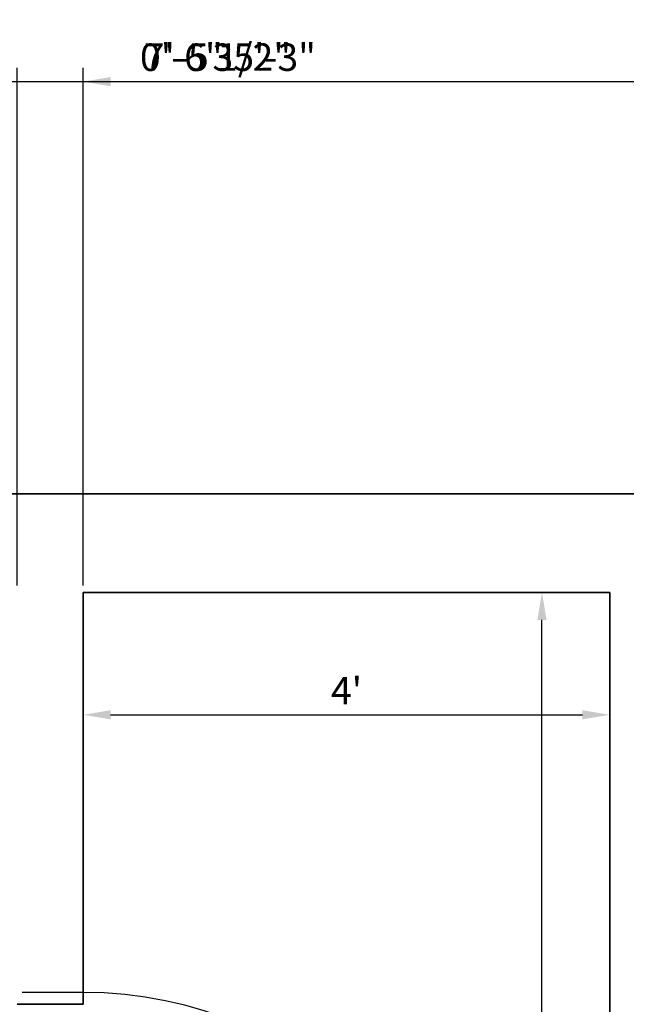
# Model space of a CAD drawing. Units: inches. Extents: x 2025 to 2528, y 1525 to 2336.
# Tile 17 of 18: x 2255 to 2311, y 2246 to 2336. Entities that reach past the tile are written whole.
import ezdxf

# ---------------------------------------------------------------- set-up
doc = ezdxf.new("R2010")
doc.units = ezdxf.units.IN
for name, color, linetype, lineweight in [('A-ANNO-DIMS', 2, 'Continuous', 18), ('A-DOOR', 3, 'Continuous', 25), ('A-WALL', 7, 'Continuous', 35)]:
    doc.layers.add(name, color=color, linetype=linetype, lineweight=lineweight)
doc.styles.get("Standard").update_dxf_attribs({"font": 'arial.ttf'})
doc.dimstyles.new('Copy of ISO-25', dxfattribs={"dimtxt": 2.5, "dimasz": 2.5, "dimexe": 1.25, "dimexo": 0.625, "dimtad": 1, "dimdec": 1, "dimlunit": 4, "dimtxsty": 'Standard', "dimcen": 2.5, "dimadec": 0, "dimazin": 0, "dimtfac": 1, "dimtdec": 1, "dimtmove": 0, "dimatfit": 3, "dimfxl": 1, "dimarcsym": 0})

# ---------------------------------------------------------------- blocks, each defined once
blk = doc.blocks.new('*U2')
for p, q in [((0, 0), (0, 6)), ((40, 0), (40, 6))]:
    blk.add_line(p, q)
blk.add_lwpolyline([(0, 0), (0, -40), (1.75, -40), (1.75, 0)], close=True)
blk.add_arc((0, 0), 40, 270, 0)
blk = doc.blocks.new('*D8')
at = {"layer": 'A-ANNO-DIMS', "color": 0, "lineweight": -2, "transparency": 16777216}
for p, q in [((2261.013, 2282.787), (2261.013, 2271.008)), ((2309.013, 2282.787), (2309.013, 2271.008)), ((2263.513, 2272.258), (2306.513, 2272.258))]:
    blk.add_line(p, q, dxfattribs=at)
at = {"layer": 'A-ANNO-DIMS', "color": 0, "transparency": 16777216}
for points in [[(2263.513, 2272.675), (2263.513, 2271.842), (2261.013, 2272.258)], [(2306.513, 2272.675), (2306.513, 2271.842), (2309.013, 2272.258)]]:
    blk.add_solid(points, dxfattribs=at)
at = {"layer": 'Defpoints', "color": 0, "transparency": 16777216}
for p in [(2261.013, 2283.412), (2309.013, 2283.412), (2309.013, 2272.258)]:
    blk.add_point(p, dxfattribs=at)
at = {"layer": 'A-ANNO-DIMS', "color": 0, "transparency": 16777216, "insert": (2285.013, 2274.133), "char_height": 2.5, "attachment_point": 5}
blk.add_mtext("4'", dxfattribs=at)
blk = doc.blocks.new('*D9')
at = {"layer": 'A-ANNO-DIMS', "color": 0, "lineweight": -2, "transparency": 16777216}
for p, q in [((2308.388, 2283.412), (2301.577, 2283.412)), ((2302.827, 2201.912), (2302.827, 2280.912)), ((2308.388, 2199.412), (2301.577, 2199.412))]:
    blk.add_line(p, q, dxfattribs=at)
at = {"layer": 'A-ANNO-DIMS', "color": 0, "transparency": 16777216}
for points in [[(2302.41, 2280.912), (2303.243, 2280.912), (2302.827, 2283.412)], [(2302.41, 2201.912), (2303.243, 2201.912), (2302.827, 2199.412)]]:
    blk.add_solid(points, dxfattribs=at)
at = {"layer": 'Defpoints', "color": 0, "transparency": 16777216}
for p in [(2302.827, 2283.412), (2309.013, 2283.412), (2309.013, 2199.412)]:
    blk.add_point(p, dxfattribs=at)
at = {"layer": 'A-ANNO-DIMS', "color": 0, "transparency": 16777216, "insert": (2300.952, 2241.412), "char_height": 2.5, "attachment_point": 5, "rotation": 90}
blk.add_mtext("7'", dxfattribs=at)
blk = doc.blocks.new('*D62')
at = {"layer": 'A-ANNO-DIMS', "color": 0, "lineweight": -2, "transparency": 16777216}
for p, q in [((2228.485, 2293.037), (2228.485, 2331.212)), ((2318.013, 2293.037), (2318.013, 2331.212)), ((2230.985, 2329.962), (2315.513, 2329.962))]:
    blk.add_line(p, q, dxfattribs=at)
at = {"layer": 'A-ANNO-DIMS', "color": 0, "transparency": 16777216}
for points in [[(2230.985, 2330.379), (2230.985, 2329.546), (2228.485, 2329.962)], [(2315.513, 2330.379), (2315.513, 2329.546), (2318.013, 2329.962)]]:
    blk.add_solid(points, dxfattribs=at)
at = {"layer": 'Defpoints', "color": 0, "transparency": 16777216}
for p in [(2318.013, 2329.962), (2228.485, 2292.412), (2318.013, 2292.412)]:
    blk.add_point(p, dxfattribs=at)
at = {"layer": 'A-ANNO-DIMS', "color": 0, "transparency": 16777216, "insert": (2273.249, 2331.88), "char_height": 2.5, "attachment_point": 5}
blk.add_mtext('7\'-5 1/2"', dxfattribs=at)
blk = doc.blocks.new('*D74')
at = {"layer": 'A-ANNO-DIMS', "color": 0, "lineweight": -2, "transparency": 16777216}
for p, q in [((2255.013, 2284.037), (2255.013, 2331.212)), ((2261.013, 2284.037), (2261.013, 2331.212)), ((2252.513, 2329.962), (2250.013, 2329.962)), ((2255.013, 2329.962), (2261.013, 2329.962)), ((2263.513, 2329.962), (2273.909, 2329.962))]:
    blk.add_line(p, q, dxfattribs=at)
at = {"layer": 'A-ANNO-DIMS', "color": 0, "transparency": 16777216}
for points in [[(2252.513, 2330.379), (2252.513, 2329.546), (2255.013, 2329.962)], [(2263.513, 2330.379), (2263.513, 2329.546), (2261.013, 2329.962)]]:
    blk.add_solid(points, dxfattribs=at)
at = {"layer": 'Defpoints', "color": 0, "transparency": 16777216}
for p in [(2261.013, 2329.962), (2255.013, 2283.412), (2261.013, 2283.412)]:
    blk.add_point(p, dxfattribs=at)
at = {"layer": 'A-ANNO-DIMS', "color": 0, "transparency": 16777216, "insert": (2269.961, 2331.864), "char_height": 2.5, "attachment_point": 5}
blk.add_mtext('0\'-6"', dxfattribs=at)
blk = doc.blocks.new('*D79')
at = {"layer": 'A-ANNO-DIMS', "color": 0, "lineweight": -2, "transparency": 16777216}
for p, q in [((2066.013, 2293.037), (2066.013, 2331.212)), ((2489.013, 2293.037), (2489.013, 2331.212)), ((2068.513, 2329.962), (2486.513, 2329.962))]:
    blk.add_line(p, q, dxfattribs=at)
at = {"layer": 'A-ANNO-DIMS', "color": 0, "transparency": 16777216}
for points in [[(2068.513, 2330.379), (2068.513, 2329.546), (2066.013, 2329.962)], [(2486.513, 2330.379), (2486.513, 2329.546), (2489.013, 2329.962)]]:
    blk.add_solid(points, dxfattribs=at)
at = {"layer": 'Defpoints', "color": 0, "transparency": 16777216}
for p in [(2489.013, 2329.962), (2066.013, 2292.412), (2489.013, 2292.412)]:
    blk.add_point(p, dxfattribs=at)
at = {"layer": 'A-ANNO-DIMS', "color": 0, "transparency": 16777216, "insert": (2277.513, 2331.865), "char_height": 2.5, "attachment_point": 5}
blk.add_mtext('35\'-3"', dxfattribs=at)
blk = doc.blocks.new('*D80')
at = {"layer": 'A-ANNO-DIMS', "color": 0, "lineweight": -2, "transparency": 16777216}
for p, q in [((2065.388, 2292.412), (2027.213, 2292.412)), ((2028.463, 1566.912), (2028.463, 2289.912)), ((2285.388, 1564.412), (2027.213, 1564.412))]:
    blk.add_line(p, q, dxfattribs=at)
at = {"layer": 'A-ANNO-DIMS', "color": 0, "transparency": 16777216}
for points in [[(2028.046, 2289.912), (2028.88, 2289.912), (2028.463, 2292.412)], [(2028.046, 1566.912), (2028.88, 1566.912), (2028.463, 1564.412)]]:
    blk.add_solid(points, dxfattribs=at)
at = {"layer": 'Defpoints', "color": 0, "transparency": 16777216}
for p in [(2028.463, 2292.412), (2066.013, 2292.412), (2286.013, 1564.412)]:
    blk.add_point(p, dxfattribs=at)
at = {"layer": 'A-ANNO-DIMS', "color": 0, "transparency": 16777216, "insert": (2026.561, 1928.412), "char_height": 2.5, "attachment_point": 5, "rotation": 90}
blk.add_mtext('60\'-8"', dxfattribs=at)

msp = doc.modelspace()

# ---------------------------------------------------------------- linework, layer by layer
at = {"layer": 'A-WALL'}
for p, q in [((2252.013, 2292.412), (2312.013, 2292.412)), ((2261.013, 2283.412), (2309.013, 2283.412)), ((2261.013, 2245.877), (2261.013, 2283.412)), ((2261.013, 2283.412), (2309.013, 2283.412)), ((2309.013, 2283.412), (2309.013, 2115.412)), ((2309.013, 2283.412), (2309.013, 2199.412)), ((2255.013, 2245.877), (2261.013, 2245.877))]:
    msp.add_line(p, q, dxfattribs=at)

# ---------------------------------------------------------------- block references
at = {"layer": 'A-DOOR', "xscale": 0.9271117355112991, "yscale": 0.9271117355112991, "zscale": 0.9271117355112991, "rotation": 90}
msp.add_blockref('*U2', (2261.013, 2209.877), dxfattribs=at)

# ---------------------------------------------------------------- dimensions: what is measured, and where the dimension line sits
at = {"layer": 'A-ANNO-DIMS'}
for base, p1, p2, override, picture, middle in [((2318.013, 2329.962), (2228.485, 2292.412), (2318.013, 2292.412), {"dimdec": 1, "dimlfac": 1, "dimrnd": 0, "dimzin": 1, "dimdsep": 46, "dimlunit": 4, "dimfrac": 2}, '*D62', (2273.249, 2331.88)), ((2489.013, 2329.962), (2066.013, 2292.412), (2489.013, 2292.412), {"dimdec": 1, "dimlfac": 1, "dimrnd": 0, "dimzin": 1, "dimdsep": 46, "dimlunit": 4, "dimfrac": 2}, '*D79', (2277.513, 2331.865)), ((2261.013, 2329.962), (2255.013, 2283.412), (2261.013, 2283.412), {"dimdec": 1, "dimlfac": 1, "dimrnd": 0, "dimzin": 1, "dimdsep": 46, "dimlunit": 4, "dimfrac": 2}, '*D74', (2269.961, 2331.864)), ((2309.013, 2272.258), (2261.013, 2283.412), (2309.013, 2283.412), {"dimclrd": 0, "dimclre": 0, "dimclrt": 0}, '*D8', (2285.013, 2274.133))]:
    dim = msp.add_linear_dim(base=base, p1=p1, p2=p2, dimstyle='Copy of ISO-25', override=override, dxfattribs=at)
    dim.commit()
    dim.dimension.update_dxf_attribs({"geometry": picture, "text_midpoint": middle})
for base, p1, p2, override, picture, middle in [((2028.463, 2292.412), (2286.013, 1564.412), (2066.013, 2292.412), {"dimdec": 1, "dimlfac": 1, "dimrnd": 0, "dimzin": 1, "dimdsep": 46, "dimlunit": 4, "dimfrac": 2}, '*D80', (2026.561, 1928.412)), ((2302.827, 2283.412), (2309.013, 2199.412), (2309.013, 2283.412), {"dimclrd": 0, "dimclre": 0, "dimclrt": 0}, '*D9', (2300.952, 2241.412))]:
    dim = msp.add_linear_dim(base=base, p1=p1, p2=p2, angle=90, dimstyle='Copy of ISO-25', override=override, dxfattribs=at)
    dim.commit()
    dim.dimension.update_dxf_attribs({"geometry": picture, "text_midpoint": middle})

doc.saveas('drawing.dxf')
